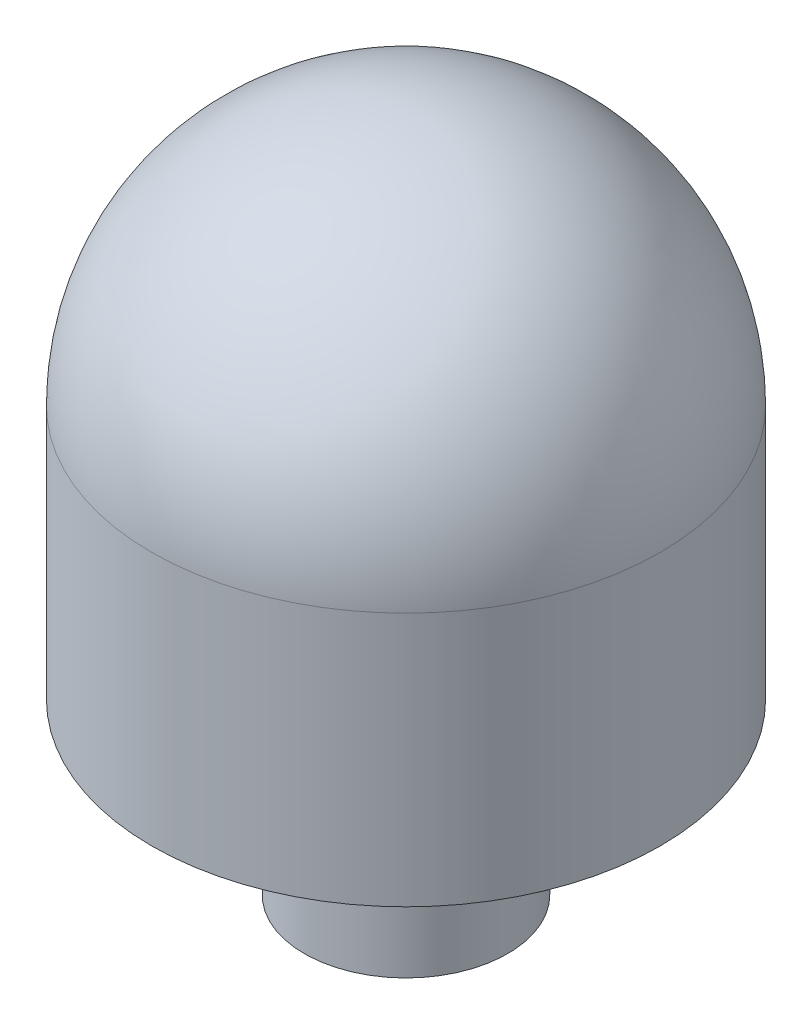
from build123d import *


with BuildPart() as part:
    # Pin Profile Sketch → Pin Body Revolve (revolve)
    with BuildSketch(Plane.XY, mode=Mode.PRIVATE) as pin_body_revolve_sk:
        with BuildLine():
            Line((0, 0), (6, 0))
            Line((6, 0), (6, 10))
            Line((6, 10), (15, 10))
            Line((15, 10), (15, 25))
            ThreePointArc((15, 25), (10.606601718, 35.606601718), (0, 40))
            Line((0, 40), (0, 0))
        make_face()
    revolve(pin_body_revolve_sk.sketch.rotate(Axis((0, 40, 0), (0, -1, 0)), 180), axis=Axis((0, 40, 0), (0, -1, 0)))


solid = part.part
